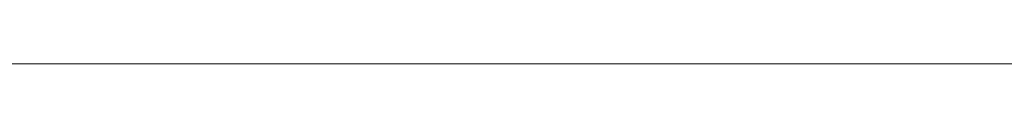
# Model space of a CAD drawing. Units: inches. Extents: x 459864 to 460310, y 324185 to 324787.
# Tile 90 of 112: x 460247.17582 to 460247.24734, y 324283.48323 to 324283.48323. Entities that reach past the tile are written whole.
import ezdxf

# ---------------------------------------------------------------- set-up
doc = ezdxf.new("R2010")
doc.units = ezdxf.units.IN
for name, color, linetype, lineweight in [('A-ANNO-DIMS', 2, 'Continuous', 18), ('L-HRDS', 9, 'Continuous', 18), ('L-SITE-PATT', 252, 'Continuous', 13)]:
    doc.layers.add(name, color=color, linetype=linetype, lineweight=lineweight)
doc.styles.get("Standard").update_dxf_attribs({"font": 'arial.ttf'})
doc.dimstyles.new('ISO-25', dxfattribs={"dimtxt": 6, "dimasz": 2.5, "dimexe": 1.25, "dimexo": 0.625, "dimtad": 1, "dimdec": 1, "dimlunit": 3, "dimtxsty": 'Standard', "dimcen": 2.5, "dimadec": 0, "dimazin": 0, "dimtfac": 1, "dimtdec": 1, "dimtmove": 0, "dimatfit": 3, "dimfxl": 1, "dimarcsym": 0})

# ---------------------------------------------------------------- blocks, each defined once
blk = doc.blocks.new('*D21')
at = {"layer": 'A-ANNO-DIMS', "color": 0, "lineweight": -2, "transparency": 16777216}
for p, q in [((460247.739927, 324715.483233), (460309.580369, 324715.483233)), ((460308.330369, 324712.983233), (460308.330369, 324285.983233)), ((460247.739927, 324283.483233), (460309.580369, 324283.483233))]:
    blk.add_line(p, q, dxfattribs=at)
at = {"layer": 'A-ANNO-DIMS', "color": 0, "transparency": 16777216}
for points in [[(460307.913702, 324712.983233), (460308.747035, 324712.983233), (460308.330369, 324715.483233)], [(460307.913702, 324285.983233), (460308.747035, 324285.983233), (460308.330369, 324283.483233)]]:
    blk.add_solid(points, dxfattribs=at)
at = {"layer": 'Defpoints', "color": 0, "transparency": 16777216}
for p in [(460247.114927, 324715.483233), (460247.114927, 324283.483233), (460308.330369, 324283.483233)]:
    blk.add_point(p, dxfattribs=at)
at = {"layer": 'A-ANNO-DIMS', "color": 0, "transparency": 16777216, "insert": (460304.639884, 324499.483233), "char_height": 6, "attachment_point": 5, "rotation": 90}
blk.add_mtext("36'", dxfattribs=at)

msp = doc.modelspace()

# ---------------------------------------------------------------- hatches: boundary and pattern name
at = {"layer": 'L-SITE-PATT'}
h = msp.add_hatch(dxfattribs=at)
h.set_pattern_fill('DOTS', color=256)
h.paths.add_polyline_path([(460269.803614, 324283.483233), (460247.114927, 324283.483233), (460121.929275, 324283.483233), (460121.929275, 324252.47302), (460117.429275, 324252.47302), (460110.123563, 324252.47302), (460110.123563, 324243.286537), (460080.829543, 324243.286537), (460080.829543, 324252.47302), (460061.114927, 324252.47302), (460061.114927, 324251.882422), (460077.9089, 324251.882422), (460077.9089, 324199.483233), (460080.829543, 324199.483233), (460080.829543, 324207.553216), (460110.123563, 324207.553216), (460110.123563, 324199.483233), (460110.813349, 324199.483233), (460262.114927, 324199.483233), (460269.803614, 324199.483233)], flags=17)
edge = h.paths.add_edge_path(flags=0)
edge.add_ellipse((460222.590295, 324263.813229), major_axis=(-8.485281, 8.485281), ratio=1, start_angle=405, end_angle=495, ccw=False)
edge.add_line((460214.820868, 324254.65989), (460214.831619, 324254.66592))
edge.add_ellipse((460222.590295, 324263.813229), major_axis=(-8.485281, 8.485281), ratio=1, start_angle=405, end_angle=495, ccw=False)
edge.add_line((460210.75891, 324261.780551), (460210.767583, 324261.786823))
edge.add_ellipse((460222.590295, 324263.813229), major_axis=(-8.485281, 8.485281), ratio=1, start_angle=405, end_angle=495, ccw=False)
edge.add_ellipse((460222.590295, 324263.813229), major_axis=(-8.485281, 8.485281), ratio=1, start_angle=392.754016, end_angle=405, ccw=False)
edge.add_ellipse((460222.590295, 324263.813229), major_axis=(-8.485281, 8.485281), ratio=1, start_angle=380.9347178, end_angle=392.754016, ccw=False)
edge.add_line((460211.337059, 324267.985029), (460211.340404, 324267.985029))
edge.add_ellipse((460222.590295, 324263.813229), major_axis=(-8.485281, 8.485281), ratio=1, start_angle=380.9347178, end_angle=392.754016, ccw=False)
edge.add_ellipse((460222.590295, 324263.813229), major_axis=(-8.485281, 8.485281), ratio=1, start_angle=347.9015209, end_angle=380.9347178, ccw=False)
edge.add_ellipse((460222.590295, 324263.813229), major_axis=(-8.485281, 8.485281), ratio=1, start_angle=327.0619241, end_angle=347.9015209, ccw=False)
edge.add_ellipse((460222.590295, 324263.813229), major_axis=(-8.485281, 8.485281), ratio=1, start_angle=278.3246418, end_angle=327.0619241, ccw=False)
edge.add_line((460225.158278, 324275.535991), (460225.157699, 324275.534637))
edge.add_ellipse((460222.590295, 324263.813229), major_axis=(-8.485281, 8.485281), ratio=1, start_angle=278.3246418, end_angle=327.0619241, ccw=False)
edge.add_ellipse((460222.590295, 324263.813229), major_axis=(-8.485281, 8.485281), ratio=1, start_angle=260.6435685, end_angle=278.3246418, ccw=False)
edge.add_ellipse((460222.590295, 324263.813229), major_axis=(-8.485281, 8.485281), ratio=1, start_angle=225, end_angle=260.6435685, ccw=False)
edge.add_line((460234.508791, 324265.242796), (460234.501456, 324265.239441))
edge.add_ellipse((460222.590295, 324263.813229), major_axis=(-8.485281, 8.485281), ratio=1, start_angle=225, end_angle=260.6435685, ccw=False)
edge.add_ellipse((460222.590295, 324263.813229), major_axis=(-8.485281, 8.485281), ratio=1, start_angle=495, end_angle=585, ccw=False)
edge.add_line((460234.436668, 324261.861215), (460234.423783, 324261.857822))
edge.add_ellipse((460222.590295, 324263.813229), major_axis=(-8.485281, 8.485281), ratio=1, start_angle=495, end_angle=585, ccw=False)
edge.add_line((460227.95013, 324253.067192), (460227.946414, 324253.083139))
edge.add_ellipse((460222.590295, 324263.813229), major_axis=(-8.485281, 8.485281), ratio=1, start_angle=495, end_angle=585, ccw=False)
edge.add_line((460226.222975, 324252.369267), (460226.21103, 324252.379551))
edge.add_ellipse((460222.590295, 324263.813229), major_axis=(-8.485281, 8.485281), ratio=1, start_angle=495, end_angle=585, ccw=False)
h.paths.add_polyline_path([(460219.651452, 324254.346654), (460218.461311, 324253.544985), (460218.275437, 324254.78932), (460219.642395, 324256.541765), (460219.62463, 324260.847564), (460216.110089, 324257.333022), (460214.349967, 324256.978066), (460215.416366, 324259.355678), (460212.523935, 324258.495823), (460213.137313, 324259.929797), (460218.507211, 324263.813229), (460222.590295, 324263.813229), (460222.590295, 324267.806698), (460218.175536, 324272.21231), (460219.025968, 324274.63898), (460222.590295, 324272.811129), (460222.590295, 324275.42332), (460223.057099, 324274.824931), (460222.67523, 324273.492211), (460225.911677, 324267.134611), (460219.62463, 324260.847564)], flags=0)
edge = h.paths.add_edge_path(flags=0)
edge.add_ellipse((460194.575758, 324264.046494), major_axis=(-8.485281, 8.485281), ratio=1, start_angle=495, end_angle=585, ccw=False)
edge.add_line((460199.935593, 324253.300458), (460199.931877, 324253.316405))
edge.add_ellipse((460194.575758, 324264.046494), major_axis=(-8.485281, 8.485281), ratio=1, start_angle=495, end_angle=585, ccw=False)
edge.add_line((460198.208438, 324252.602533), (460198.196493, 324252.612817))
edge.add_ellipse((460194.575758, 324264.046494), major_axis=(-8.485281, 8.485281), ratio=1, start_angle=495, end_angle=585, ccw=False)
edge.add_ellipse((460194.575758, 324264.046494), major_axis=(-8.485281, 8.485281), ratio=1, start_angle=405, end_angle=495, ccw=False)
edge.add_line((460186.806331, 324254.893156), (460186.817082, 324254.899186))
edge.add_ellipse((460194.575758, 324264.046494), major_axis=(-8.485281, 8.485281), ratio=1, start_angle=405, end_angle=495, ccw=False)
edge.add_line((460182.744373, 324262.013817), (460182.753046, 324262.020089))
edge.add_ellipse((460194.575758, 324264.046494), major_axis=(-8.485281, 8.485281), ratio=1, start_angle=405, end_angle=495, ccw=False)
edge.add_ellipse((460194.575758, 324264.046494), major_axis=(-8.485281, 8.485281), ratio=1, start_angle=392.754016, end_angle=405, ccw=False)
edge.add_ellipse((460194.575758, 324264.046494), major_axis=(-8.485281, 8.485281), ratio=1, start_angle=380.9347178, end_angle=392.754016, ccw=False)
edge.add_line((460183.322522, 324268.218294), (460183.325867, 324268.218294))
edge.add_ellipse((460194.575758, 324264.046494), major_axis=(-8.485281, 8.485281), ratio=1, start_angle=380.9347178, end_angle=392.754016, ccw=False)
edge.add_ellipse((460194.575758, 324264.046494), major_axis=(-8.485281, 8.485281), ratio=1, start_angle=347.9015209, end_angle=380.9347178, ccw=False)
edge.add_ellipse((460194.575758, 324264.046494), major_axis=(-8.485281, 8.485281), ratio=1, start_angle=327.0619241, end_angle=347.9015209, ccw=False)
edge.add_ellipse((460194.575758, 324264.046494), major_axis=(-8.485281, 8.485281), ratio=1, start_angle=278.3246418, end_angle=327.0619241, ccw=False)
edge.add_line((460197.143741, 324275.769257), (460197.143162, 324275.767903))
edge.add_ellipse((460194.575758, 324264.046494), major_axis=(-8.485281, 8.485281), ratio=1, start_angle=278.3246418, end_angle=327.0619241, ccw=False)
edge.add_ellipse((460194.575758, 324264.046494), major_axis=(-8.485281, 8.485281), ratio=1, start_angle=260.6435685, end_angle=278.3246418, ccw=False)
edge.add_ellipse((460194.575758, 324264.046494), major_axis=(-8.485281, 8.485281), ratio=1, start_angle=225, end_angle=260.6435685, ccw=False)
edge.add_line((460206.494254, 324265.476062), (460206.486919, 324265.472707))
edge.add_ellipse((460194.575758, 324264.046494), major_axis=(-8.485281, 8.485281), ratio=1, start_angle=225, end_angle=260.6435685, ccw=False)
edge.add_ellipse((460194.575758, 324264.046494), major_axis=(-8.485281, 8.485281), ratio=1, start_angle=495, end_angle=585, ccw=False)
edge.add_line((460206.422132, 324262.094481), (460206.409246, 324262.091088))
h.paths.add_polyline_path([(460191.610093, 324261.08083), (460191.636915, 324254.57992), (460190.446774, 324253.778251), (460190.2609, 324255.022585), (460191.627858, 324256.775031), (460191.610093, 324261.08083), (460188.095552, 324257.566288), (460186.33543, 324257.211332), (460187.40183, 324259.588944), (460184.509398, 324258.729088), (460185.122776, 324260.163063), (460190.492675, 324264.046494), (460194.575758, 324264.046494), (460194.575758, 324268.039963), (460190.160999, 324272.445576), (460191.011431, 324274.872246), (460194.575758, 324273.044395), (460194.575758, 324275.656585), (460195.042562, 324275.058197), (460194.660693, 324273.725477), (460197.897141, 324267.367877)], flags=0)
edge = h.paths.add_edge_path(flags=0)
edge.add_ellipse((460252.911961, 324263.577616), major_axis=(-8.485281, 8.485281), ratio=1, start_angle=405, end_angle=495, ccw=False)
edge.add_line((460241.080576, 324261.544938), (460241.089249, 324261.55121))
edge.add_ellipse((460252.911961, 324263.577616), major_axis=(-8.485281, 8.485281), ratio=1, start_angle=405, end_angle=495, ccw=False)
edge.add_ellipse((460252.911961, 324263.577616), major_axis=(-8.485281, 8.485281), ratio=1, start_angle=392.754016, end_angle=405, ccw=False)
edge.add_ellipse((460252.911961, 324263.577616), major_axis=(-8.485281, 8.485281), ratio=1, start_angle=380.9347178, end_angle=392.754016, ccw=False)
edge.add_line((460241.658725, 324267.749416), (460241.66207, 324267.749416))
edge.add_ellipse((460252.911961, 324263.577616), major_axis=(-8.485281, 8.485281), ratio=1, start_angle=380.9347178, end_angle=392.754016, ccw=False)
edge.add_ellipse((460252.911961, 324263.577616), major_axis=(-8.485281, 8.485281), ratio=1, start_angle=347.9015209, end_angle=380.9347178, ccw=False)
edge.add_ellipse((460252.911961, 324263.577616), major_axis=(-8.485281, 8.485281), ratio=1, start_angle=327.0619241, end_angle=347.9015209, ccw=False)
edge.add_ellipse((460252.911961, 324263.577616), major_axis=(-8.485281, 8.485281), ratio=1, start_angle=278.3246418, end_angle=327.0619241, ccw=False)
edge.add_line((460255.479944, 324275.300378), (460255.479365, 324275.299024))
edge.add_ellipse((460252.911961, 324263.577616), major_axis=(-8.485281, 8.485281), ratio=1, start_angle=278.3246418, end_angle=327.0619241, ccw=False)
edge.add_ellipse((460252.911961, 324263.577616), major_axis=(-8.485281, 8.485281), ratio=1, start_angle=260.6435685, end_angle=278.3246418, ccw=False)
edge.add_ellipse((460252.911961, 324263.577616), major_axis=(-8.485281, 8.485281), ratio=1, start_angle=225, end_angle=260.6435685, ccw=False)
edge.add_line((460264.830457, 324265.007183), (460264.823122, 324265.003828))
edge.add_ellipse((460252.911961, 324263.577616), major_axis=(-8.485281, 8.485281), ratio=1, start_angle=225, end_angle=260.6435685, ccw=False)
edge.add_ellipse((460252.911961, 324263.577616), major_axis=(-8.485281, 8.485281), ratio=1, start_angle=495, end_angle=585, ccw=False)
edge.add_line((460264.758335, 324261.625602), (460264.745449, 324261.622209))
edge.add_ellipse((460252.911961, 324263.577616), major_axis=(-8.485281, 8.485281), ratio=1, start_angle=495, end_angle=585, ccw=False)
edge.add_line((460258.271796, 324252.831579), (460258.268081, 324252.847526))
edge.add_ellipse((460252.911961, 324263.577616), major_axis=(-8.485281, 8.485281), ratio=1, start_angle=495, end_angle=585, ccw=False)
edge.add_line((460256.544641, 324252.133654), (460256.532696, 324252.143938))
edge.add_ellipse((460252.911961, 324263.577616), major_axis=(-8.485281, 8.485281), ratio=1, start_angle=495, end_angle=585, ccw=False)
edge.add_ellipse((460252.911961, 324263.577616), major_axis=(-8.485281, 8.485281), ratio=1, start_angle=405, end_angle=495, ccw=False)
edge.add_line((460245.142534, 324254.424277), (460245.153285, 324254.430307))
h.paths.add_polyline_path([(460244.671633, 324256.742453), (460245.738033, 324259.120065), (460242.845601, 324258.26021), (460243.458979, 324259.694184), (460248.828878, 324263.577616), (460252.911961, 324263.577616), (460252.911961, 324267.571085), (460248.497202, 324271.976697), (460249.347634, 324274.403367), (460252.911961, 324272.575516), (460252.911961, 324275.187707), (460253.378765, 324274.589318), (460252.996897, 324273.256598), (460256.233344, 324266.898998), (460249.946296, 324260.611951), (460249.973118, 324254.111041), (460248.782977, 324253.309372), (460248.597103, 324254.553707), (460249.964061, 324256.306152), (460249.946296, 324260.611951), (460246.431755, 324257.097409)], flags=0)
edge = h.paths.add_edge_path(flags=0)
edge.add_ellipse((460167.43869, 324262.832792), major_axis=(-8.485281, 8.485281), ratio=1, start_angle=495, end_angle=585, ccw=False)
edge.add_line((460172.798524, 324252.086755), (460172.794809, 324252.102702))
edge.add_ellipse((460167.43869, 324262.832792), major_axis=(-8.485281, 8.485281), ratio=1, start_angle=495, end_angle=585, ccw=False)
edge.add_line((460171.07137, 324251.38883), (460171.059425, 324251.399114))
edge.add_ellipse((460167.43869, 324262.832792), major_axis=(-8.485281, 8.485281), ratio=1, start_angle=495, end_angle=585, ccw=False)
edge.add_ellipse((460167.43869, 324262.832792), major_axis=(-8.485281, 8.485281), ratio=1, start_angle=405, end_angle=495, ccw=False)
edge.add_line((460159.669262, 324253.679453), (460159.680013, 324253.685483))
edge.add_ellipse((460167.43869, 324262.832792), major_axis=(-8.485281, 8.485281), ratio=1, start_angle=405, end_angle=495, ccw=False)
edge.add_line((460155.607304, 324260.800114), (460155.615977, 324260.806386))
edge.add_ellipse((460167.43869, 324262.832792), major_axis=(-8.485281, 8.485281), ratio=1, start_angle=405, end_angle=495, ccw=False)
edge.add_ellipse((460167.43869, 324262.832792), major_axis=(-8.485281, 8.485281), ratio=1, start_angle=392.754016, end_angle=405, ccw=False)
edge.add_ellipse((460167.43869, 324262.832792), major_axis=(-8.485281, 8.485281), ratio=1, start_angle=380.9347178, end_angle=392.754016, ccw=False)
edge.add_line((460156.185453, 324267.004592), (460156.188798, 324267.004592))
edge.add_ellipse((460167.43869, 324262.832792), major_axis=(-8.485281, 8.485281), ratio=1, start_angle=380.9347178, end_angle=392.754016, ccw=False)
edge.add_ellipse((460167.43869, 324262.832792), major_axis=(-8.485281, 8.485281), ratio=1, start_angle=347.9015209, end_angle=380.9347178, ccw=False)
edge.add_ellipse((460167.43869, 324262.832792), major_axis=(-8.485281, 8.485281), ratio=1, start_angle=327.0619241, end_angle=347.9015209, ccw=False)
edge.add_ellipse((460167.43869, 324262.832792), major_axis=(-8.485281, 8.485281), ratio=1, start_angle=278.3246418, end_angle=327.0619241, ccw=False)
edge.add_line((460170.006672, 324274.555554), (460170.006093, 324274.5542))
edge.add_ellipse((460167.43869, 324262.832792), major_axis=(-8.485281, 8.485281), ratio=1, start_angle=278.3246418, end_angle=327.0619241, ccw=False)
edge.add_ellipse((460167.43869, 324262.832792), major_axis=(-8.485281, 8.485281), ratio=1, start_angle=260.6435685, end_angle=278.3246418, ccw=False)
edge.add_ellipse((460167.43869, 324262.832792), major_axis=(-8.485281, 8.485281), ratio=1, start_angle=225, end_angle=260.6435685, ccw=False)
edge.add_line((460179.357186, 324264.262359), (460179.349851, 324264.259004))
edge.add_ellipse((460167.43869, 324262.832792), major_axis=(-8.485281, 8.485281), ratio=1, start_angle=225, end_angle=260.6435685, ccw=False)
edge.add_ellipse((460167.43869, 324262.832792), major_axis=(-8.485281, 8.485281), ratio=1, start_angle=495, end_angle=585, ccw=False)
edge.add_line((460179.285063, 324260.880778), (460179.272177, 324260.877385))
h.paths.add_polyline_path([(460164.473025, 324259.867127), (460164.499846, 324253.366217), (460163.309706, 324252.564548), (460163.123831, 324253.808883), (460164.49079, 324255.561328), (460164.473025, 324259.867127), (460160.958483, 324256.352585), (460159.198362, 324255.997629), (460160.264761, 324258.375241), (460157.372329, 324257.515386), (460157.985707, 324258.94936), (460163.355606, 324262.832792), (460167.43869, 324262.832792), (460167.43869, 324266.826261), (460163.02393, 324271.231873), (460163.874362, 324273.658543), (460167.43869, 324271.830692), (460167.43869, 324274.442883), (460167.905493, 324273.844494), (460167.523625, 324272.511774), (460170.760072, 324266.154174)], flags=0)
edge = h.paths.add_edge_path(flags=0)
edge.add_ellipse((460140.758089, 324262.369585), major_axis=(-8.485281, 8.485281), ratio=1, start_angle=495, end_angle=585, ccw=False)
edge.add_line((460146.117923, 324251.623548), (460146.114208, 324251.639495))
edge.add_ellipse((460140.758089, 324262.369585), major_axis=(-8.485281, 8.485281), ratio=1, start_angle=495, end_angle=585, ccw=False)
edge.add_line((460144.390769, 324250.925623), (460144.378824, 324250.935907))
edge.add_ellipse((460140.758089, 324262.369585), major_axis=(-8.485281, 8.485281), ratio=1, start_angle=495, end_angle=585, ccw=False)
edge.add_ellipse((460140.758089, 324262.369585), major_axis=(-8.485281, 8.485281), ratio=1, start_angle=405, end_angle=495, ccw=False)
edge.add_line((460132.988661, 324253.216246), (460132.999412, 324253.222276))
edge.add_ellipse((460140.758089, 324262.369585), major_axis=(-8.485281, 8.485281), ratio=1, start_angle=405, end_angle=495, ccw=False)
edge.add_line((460128.926703, 324260.336907), (460128.935376, 324260.343179))
edge.add_ellipse((460140.758089, 324262.369585), major_axis=(-8.485281, 8.485281), ratio=1, start_angle=405, end_angle=495, ccw=False)
edge.add_ellipse((460140.758089, 324262.369585), major_axis=(-8.485281, 8.485281), ratio=1, start_angle=392.754016, end_angle=405, ccw=False)
edge.add_ellipse((460140.758089, 324262.369585), major_axis=(-8.485281, 8.485281), ratio=1, start_angle=380.9347178, end_angle=392.754016, ccw=False)
edge.add_line((460129.504852, 324266.541385), (460129.508197, 324266.541385))
edge.add_ellipse((460140.758089, 324262.369585), major_axis=(-8.485281, 8.485281), ratio=1, start_angle=380.9347178, end_angle=392.754016, ccw=False)
edge.add_ellipse((460140.758089, 324262.369585), major_axis=(-8.485281, 8.485281), ratio=1, start_angle=347.9015209, end_angle=380.9347178, ccw=False)
edge.add_ellipse((460140.758089, 324262.369585), major_axis=(-8.485281, 8.485281), ratio=1, start_angle=327.0619241, end_angle=347.9015209, ccw=False)
edge.add_ellipse((460140.758089, 324262.369585), major_axis=(-8.485281, 8.485281), ratio=1, start_angle=278.3246418, end_angle=327.0619241, ccw=False)
edge.add_line((460143.326071, 324274.092347), (460143.325492, 324274.090993))
edge.add_ellipse((460140.758089, 324262.369585), major_axis=(-8.485281, 8.485281), ratio=1, start_angle=278.3246418, end_angle=327.0619241, ccw=False)
edge.add_ellipse((460140.758089, 324262.369585), major_axis=(-8.485281, 8.485281), ratio=1, start_angle=260.6435685, end_angle=278.3246418, ccw=False)
edge.add_ellipse((460140.758089, 324262.369585), major_axis=(-8.485281, 8.485281), ratio=1, start_angle=225, end_angle=260.6435685, ccw=False)
edge.add_line((460152.676585, 324263.799152), (460152.66925, 324263.795797))
edge.add_ellipse((460140.758089, 324262.369585), major_axis=(-8.485281, 8.485281), ratio=1, start_angle=225, end_angle=260.6435685, ccw=False)
edge.add_ellipse((460140.758089, 324262.369585), major_axis=(-8.485281, 8.485281), ratio=1, start_angle=495, end_angle=585, ccw=False)
edge.add_line((460152.604462, 324260.417571), (460152.591576, 324260.414178))
h.paths.add_polyline_path([(460137.792424, 324259.40392), (460137.819245, 324252.90301), (460136.629105, 324252.101341), (460136.44323, 324253.345676), (460137.810189, 324255.098121), (460137.792424, 324259.40392), (460134.277882, 324255.889378), (460132.517761, 324255.534422), (460133.58416, 324257.912034), (460130.691728, 324257.052179), (460131.305106, 324258.486153), (460136.675005, 324262.369585), (460140.758089, 324262.369585), (460140.758089, 324266.363054), (460136.343329, 324270.768666), (460137.193761, 324273.195336), (460140.758089, 324271.367485), (460140.758089, 324273.979676), (460141.224892, 324273.381287), (460140.843024, 324272.048567), (460144.079471, 324265.690967)], flags=0)
h.paths.add_polyline_path([(460110.123563, 324227.413868), (460080.829543, 324227.413868), (460080.829543, 324235.483851), (460110.123563, 324235.483851)], flags=16)
h.paths.add_polyline_path([(460110.123563, 324220.796634), (460110.123563, 324212.726651), (460080.829543, 324212.726651), (460080.829543, 324220.796634)], flags=16)
h.paths.add_polyline_path([(460269.803614, 324283.483233), (460247.114927, 324283.483233), (460121.929275, 324283.483233), (460121.929275, 324252.47302), (460117.429275, 324252.47302), (460110.123563, 324252.47302), (460110.123563, 324243.286537), (460080.829543, 324243.286537), (460080.829543, 324252.47302), (460061.114927, 324252.47302), (460061.114927, 324251.882422), (460077.9089, 324251.882422), (460077.9089, 324199.483233), (460080.829543, 324199.483233), (460080.829543, 324207.553216), (460110.123563, 324207.553216), (460110.123563, 324199.483233), (460262.114927, 324199.483233), (460269.803614, 324199.483233)], flags=17)
h.paths.add_polyline_path([(460219.651452, 324254.346654), (460218.461311, 324253.544985), (460218.275437, 324254.78932), (460219.642395, 324256.541765), (460219.62463, 324260.847564), (460216.110089, 324257.333022), (460214.349967, 324256.978066), (460215.416366, 324259.355678), (460212.523935, 324258.495823), (460213.137313, 324259.929797), (460218.507211, 324263.813229), (460222.590295, 324263.813229), (460220.180486, 324266.223037), (460215.460959, 324265.307646), (460211.834533, 324266.136551), (460216.246619, 324267.985029), (460218.418495, 324267.985029), (460222.590295, 324263.813229), (460222.590295, 324267.806698), (460218.175536, 324272.21231), (460219.025968, 324274.63898), (460222.590295, 324272.811129), (460222.590295, 324275.42332), (460223.057099, 324274.824931), (460222.67523, 324273.492211), (460225.911677, 324267.134611), (460222.590295, 324263.813229), (460231.382871, 324263.813229), (460228.484718, 324262.487825), (460224.425208, 324261.978316), (460228.679899, 324257.723625), (460228.965835, 324254.791014), (460227.141768, 324256.536632), (460227.542067, 324254.818575), (460227.333342, 324253.614466), (460222.590295, 324259.984626), (460222.590295, 324255.496666), (460221.377409, 324256.540849), (460220.575794, 324261.798728), (460219.62463, 324260.847564)], flags=0)
h.paths.add_polyline_path([(460199.127231, 324256.769898), (460199.52753, 324255.051841), (460199.318805, 324253.847732), (460194.575758, 324260.217892), (460194.575758, 324255.729932), (460193.362872, 324256.774115), (460192.561257, 324262.031993), (460191.610093, 324261.08083), (460191.636915, 324254.57992), (460190.446774, 324253.778251), (460190.2609, 324255.022585), (460191.627858, 324256.775031), (460191.610093, 324261.08083), (460188.095552, 324257.566288), (460186.33543, 324257.211332), (460187.40183, 324259.588944), (460184.509398, 324258.729088), (460185.122776, 324260.163063), (460190.492675, 324264.046494), (460194.575758, 324264.046494), (460192.16595, 324266.456303), (460187.446422, 324265.540912), (460183.819996, 324266.369816), (460188.232082, 324268.218294), (460190.403958, 324268.218294), (460194.575758, 324264.046494), (460194.575758, 324268.039963), (460190.160999, 324272.445576), (460191.011431, 324274.872246), (460194.575758, 324273.044395), (460194.575758, 324275.656585), (460195.042562, 324275.058197), (460194.660693, 324273.725477), (460197.897141, 324267.367877), (460194.575758, 324264.046494), (460203.368334, 324264.046494), (460200.470181, 324262.721091), (460196.410671, 324262.211582), (460200.665362, 324257.956891), (460200.951298, 324255.02428)], flags=0)
h.paths.add_polyline_path([(460244.671633, 324256.742453), (460245.738033, 324259.120065), (460242.845601, 324258.26021), (460243.458979, 324259.694184), (460248.828878, 324263.577616), (460252.911961, 324263.577616), (460250.502153, 324265.987424), (460245.782625, 324265.072033), (460242.156199, 324265.900938), (460246.568285, 324267.749416), (460248.740161, 324267.749416), (460252.911961, 324263.577616), (460252.911961, 324267.571085), (460248.497202, 324271.976697), (460249.347634, 324274.403367), (460252.911961, 324272.575516), (460252.911961, 324275.187707), (460253.378765, 324274.589318), (460252.996897, 324273.256598), (460256.233344, 324266.898998), (460252.911961, 324263.577616), (460261.704537, 324263.577616), (460258.806384, 324262.252212), (460254.746874, 324261.742703), (460259.001565, 324257.488012), (460259.287501, 324254.555401), (460257.463434, 324256.301019), (460257.863733, 324254.582962), (460257.655008, 324253.378853), (460252.911961, 324259.749013), (460252.911961, 324255.261053), (460251.699075, 324256.305236), (460250.89746, 324261.563115), (460249.946296, 324260.611951), (460249.973118, 324254.111041), (460248.782977, 324253.309372), (460248.597103, 324254.553707), (460249.964061, 324256.306152), (460249.946296, 324260.611951), (460246.431755, 324257.097409)], flags=0)
h.paths.add_polyline_path([(460173.528293, 324256.743188), (460173.81423, 324253.810577), (460171.990163, 324255.556195), (460172.390461, 324253.838138), (460172.181736, 324252.634029), (460167.43869, 324259.004189), (460167.43869, 324254.516229), (460166.225803, 324255.560412), (460165.424189, 324260.818291), (460164.473025, 324259.867127), (460164.499846, 324253.366217), (460163.309706, 324252.564548), (460163.123831, 324253.808883), (460164.49079, 324255.561328), (460164.473025, 324259.867127), (460160.958483, 324256.352585), (460159.198362, 324255.997629), (460160.264761, 324258.375241), (460157.372329, 324257.515386), (460157.985707, 324258.94936), (460163.355606, 324262.832792), (460167.43869, 324262.832792), (460165.028881, 324265.2426), (460160.309353, 324264.327209), (460156.682927, 324265.156114), (460161.095013, 324267.004592), (460163.26689, 324267.004592), (460167.43869, 324262.832792), (460167.43869, 324266.826261), (460163.02393, 324271.231873), (460163.874362, 324273.658543), (460167.43869, 324271.830692), (460167.43869, 324274.442883), (460167.905493, 324273.844494), (460167.523625, 324272.511774), (460170.760072, 324266.154174), (460167.43869, 324262.832792), (460176.231266, 324262.832792), (460173.333113, 324261.507388), (460169.273603, 324260.997879)], flags=0)
h.paths.add_polyline_path([(460146.847692, 324256.279981), (460147.133629, 324253.34737), (460145.309562, 324255.092988), (460145.70986, 324253.374931), (460145.501135, 324252.170822), (460140.758089, 324258.540983), (460140.758089, 324254.053022), (460139.545202, 324255.097205), (460138.743588, 324260.355084), (460137.792424, 324259.40392), (460137.819245, 324252.90301), (460136.629105, 324252.101341), (460136.44323, 324253.345676), (460137.810189, 324255.098121), (460137.792424, 324259.40392), (460134.277882, 324255.889378), (460132.517761, 324255.534422), (460133.58416, 324257.912034), (460130.691728, 324257.052179), (460131.305106, 324258.486153), (460136.675005, 324262.369585), (460140.758089, 324262.369585), (460138.34828, 324264.779393), (460133.628752, 324263.864002), (460130.002326, 324264.692907), (460134.414412, 324266.541385), (460136.586289, 324266.541385), (460140.758089, 324262.369585), (460140.758089, 324266.363054), (460136.343329, 324270.768666), (460137.193761, 324273.195336), (460140.758089, 324271.367485), (460140.758089, 324273.979676), (460141.224892, 324273.381287), (460140.843024, 324272.048567), (460144.079471, 324265.690967), (460140.758089, 324262.369585), (460149.550664, 324262.369585), (460146.652512, 324261.044182), (460142.593002, 324260.534672)], flags=0)
edge = h.paths.add_edge_path()
edge.add_line((460269.803614, 324272.549054), (460260.881484, 324272.549054))
edge.add_ellipse((460252.911961, 324263.577616), major_axis=(-8.485281, 8.485281), ratio=1, start_angle=260.6435685, end_angle=273.3846244, ccw=False)
edge.add_line((460262.282614, 324271.092108), (460262.260554, 324271.09106))
edge.add_ellipse((460252.911961, 324263.577616), major_axis=(-8.485281, 8.485281), ratio=1, start_angle=260.6435685, end_angle=273.3846244, ccw=False)
edge.add_ellipse((460252.911961, 324263.577616), major_axis=(-8.485281, 8.485281), ratio=1, start_angle=225, end_angle=260.6435685, ccw=False)
edge.add_line((460263.608568, 324269.063294), (460263.571652, 324269.058283))
edge.add_ellipse((460252.911961, 324263.577616), major_axis=(-8.485281, 8.485281), ratio=1, start_angle=225, end_angle=260.6435685, ccw=False)
edge.add_line((460264.615462, 324266.30554), (460264.585358, 324266.305196))
edge.add_ellipse((460252.911961, 324263.577616), major_axis=(-8.485281, 8.485281), ratio=1, start_angle=225, end_angle=260.6435685, ccw=False)
edge.add_line((460264.830457, 324265.007183), (460264.823122, 324265.003828))
edge.add_ellipse((460252.911961, 324263.577616), major_axis=(-8.485281, 8.485281), ratio=1, start_angle=225, end_angle=260.6435685, ccw=False)
edge.add_ellipse((460252.911961, 324263.577616), major_axis=(-8.485281, 8.485281), ratio=1, start_angle=495, end_angle=585, ccw=False)
edge.add_line((460264.758335, 324261.625602), (460264.745449, 324261.622209))
edge.add_ellipse((460252.911961, 324263.577616), major_axis=(-8.485281, 8.485281), ratio=1, start_angle=495, end_angle=585, ccw=False)
edge.add_line((460263.442202, 324257.739018), (460263.389259, 324257.779239))
edge.add_ellipse((460252.911961, 324263.577616), major_axis=(-8.485281, 8.485281), ratio=1, start_angle=495, end_angle=585, ccw=False)
edge.add_line((460258.128071, 324252.743505), (460258.101878, 324252.778683))
edge.add_ellipse((460252.911961, 324263.577616), major_axis=(-8.485281, 8.485281), ratio=1, start_angle=495, end_angle=585, ccw=False)
edge.add_line((460256.544641, 324252.133654), (460256.532696, 324252.143938))
edge.add_ellipse((460252.911961, 324263.577616), major_axis=(-8.485281, 8.485281), ratio=1, start_angle=495, end_angle=585, ccw=False)
edge.add_ellipse((460252.911961, 324263.577616), major_axis=(-8.485281, 8.485281), ratio=1, start_angle=405, end_angle=495, ccw=False)
edge.add_line((460250.593989, 324251.780412), (460250.604653, 324251.819817))
edge.add_ellipse((460252.911961, 324263.577616), major_axis=(-8.485281, 8.485281), ratio=1, start_angle=405, end_angle=495, ccw=False)
edge.add_line((460245.142534, 324254.424277), (460245.153285, 324254.430307))
edge.add_ellipse((460252.911961, 324263.577616), major_axis=(-8.485281, 8.485281), ratio=1, start_angle=405, end_angle=495, ccw=False)
edge.add_line((460243.524588, 324256.059004), (460243.560343, 324256.091361))
edge.add_ellipse((460252.911961, 324263.577616), major_axis=(-8.485281, 8.485281), ratio=1, start_angle=405, end_angle=495, ccw=False)
edge.add_line((460241.440103, 324259.892726), (460241.522441, 324259.895877))
edge.add_ellipse((460252.911961, 324263.577616), major_axis=(-8.485281, 8.485281), ratio=1, start_angle=405, end_angle=495, ccw=False)
edge.add_line((460241.080576, 324261.544938), (460241.089249, 324261.55121))
edge.add_ellipse((460252.911961, 324263.577616), major_axis=(-8.485281, 8.485281), ratio=1, start_angle=405, end_angle=495, ccw=False)
edge.add_ellipse((460252.911961, 324263.577616), major_axis=(-8.485281, 8.485281), ratio=1, start_angle=392.754016, end_angle=405, ccw=False)
edge.add_line((460241.050299, 324265.437612), (460241.062566, 324265.442751))
edge.add_ellipse((460252.911961, 324263.577616), major_axis=(-8.485281, 8.485281), ratio=1, start_angle=392.754016, end_angle=405, ccw=False)
edge.add_ellipse((460252.911961, 324263.577616), major_axis=(-8.485281, 8.485281), ratio=1, start_angle=380.9347178, end_angle=392.754016, ccw=False)
edge.add_line((460241.451888, 324267.176391), (460241.469044, 324267.170988))
edge.add_ellipse((460252.911961, 324263.577616), major_axis=(-8.485281, 8.485281), ratio=1, start_angle=380.9347178, end_angle=392.754016, ccw=False)
edge.add_line((460241.658725, 324267.749416), (460241.66207, 324267.749416))
edge.add_ellipse((460252.911961, 324263.577616), major_axis=(-8.485281, 8.485281), ratio=1, start_angle=380.9347178, end_angle=392.754016, ccw=False)
edge.add_ellipse((460252.911961, 324263.577616), major_axis=(-8.485281, 8.485281), ratio=1, start_angle=356.6153756, end_angle=380.9347178, ccw=False)
edge.add_line((460244.880293, 324272.487651), (460244.712651, 324272.549054))
edge.add_line((460244.712651, 324272.549054), (460230.817406, 324272.549054))
edge.add_ellipse((460222.590295, 324263.813229), major_axis=(-8.485281, 8.485281), ratio=1, start_angle=260.6435685, end_angle=271.7177746, ccw=False)
edge.add_ellipse((460222.590295, 324263.813229), major_axis=(-8.485281, 8.485281), ratio=1, start_angle=225, end_angle=260.6435685, ccw=False)
edge.add_line((460233.286902, 324269.298907), (460233.249986, 324269.293896))
edge.add_ellipse((460222.590295, 324263.813229), major_axis=(-8.485281, 8.485281), ratio=1, start_angle=225, end_angle=260.6435685, ccw=False)
edge.add_line((460234.293796, 324266.541153), (460234.263692, 324266.540809))
edge.add_ellipse((460222.590295, 324263.813229), major_axis=(-8.485281, 8.485281), ratio=1, start_angle=225, end_angle=260.6435685, ccw=False)
edge.add_line((460234.508791, 324265.242796), (460234.501456, 324265.239441))
edge.add_ellipse((460222.590295, 324263.813229), major_axis=(-8.485281, 8.485281), ratio=1, start_angle=225, end_angle=260.6435685, ccw=False)
edge.add_ellipse((460222.590295, 324263.813229), major_axis=(-8.485281, 8.485281), ratio=1, start_angle=495, end_angle=585, ccw=False)
edge.add_line((460234.436668, 324261.861215), (460234.423783, 324261.857822))
edge.add_ellipse((460222.590295, 324263.813229), major_axis=(-8.485281, 8.485281), ratio=1, start_angle=495, end_angle=585, ccw=False)
edge.add_line((460233.120535, 324257.974631), (460233.067593, 324258.014852))
edge.add_ellipse((460222.590295, 324263.813229), major_axis=(-8.485281, 8.485281), ratio=1, start_angle=495, end_angle=585, ccw=False)
edge.add_line((460227.806405, 324252.979118), (460227.780212, 324253.014296))
edge.add_ellipse((460222.590295, 324263.813229), major_axis=(-8.485281, 8.485281), ratio=1, start_angle=495, end_angle=585, ccw=False)
edge.add_line((460226.222975, 324252.369267), (460226.21103, 324252.379551))
edge.add_ellipse((460222.590295, 324263.813229), major_axis=(-8.485281, 8.485281), ratio=1, start_angle=495, end_angle=585, ccw=False)
edge.add_ellipse((460222.590295, 324263.813229), major_axis=(-8.485281, 8.485281), ratio=1, start_angle=405, end_angle=495, ccw=False)
edge.add_line((460220.272323, 324252.016025), (460220.282987, 324252.05543))
edge.add_ellipse((460222.590295, 324263.813229), major_axis=(-8.485281, 8.485281), ratio=1, start_angle=405, end_angle=495, ccw=False)
edge.add_line((460214.820868, 324254.65989), (460214.831619, 324254.66592))
edge.add_ellipse((460222.590295, 324263.813229), major_axis=(-8.485281, 8.485281), ratio=1, start_angle=405, end_angle=495, ccw=False)
edge.add_line((460213.202922, 324256.294617), (460213.238677, 324256.326974))
edge.add_ellipse((460222.590295, 324263.813229), major_axis=(-8.485281, 8.485281), ratio=1, start_angle=405, end_angle=495, ccw=False)
edge.add_line((460211.118437, 324260.128339), (460211.200774, 324260.13149))
edge.add_ellipse((460222.590295, 324263.813229), major_axis=(-8.485281, 8.485281), ratio=1, start_angle=405, end_angle=495, ccw=False)
edge.add_line((460210.75891, 324261.780551), (460210.767583, 324261.786823))
edge.add_ellipse((460222.590295, 324263.813229), major_axis=(-8.485281, 8.485281), ratio=1, start_angle=405, end_angle=495, ccw=False)
edge.add_ellipse((460222.590295, 324263.813229), major_axis=(-8.485281, 8.485281), ratio=1, start_angle=392.754016, end_angle=405, ccw=False)
edge.add_line((460210.728633, 324265.673225), (460210.7409, 324265.678364))
edge.add_ellipse((460222.590295, 324263.813229), major_axis=(-8.485281, 8.485281), ratio=1, start_angle=392.754016, end_angle=405, ccw=False)
edge.add_ellipse((460222.590295, 324263.813229), major_axis=(-8.485281, 8.485281), ratio=1, start_angle=380.9347178, end_angle=392.754016, ccw=False)
edge.add_line((460211.130222, 324267.412004), (460211.147378, 324267.406601))
edge.add_ellipse((460222.590295, 324263.813229), major_axis=(-8.485281, 8.485281), ratio=1, start_angle=380.9347178, end_angle=392.754016, ccw=False)
edge.add_line((460211.337059, 324267.985029), (460211.340404, 324267.985029))
edge.add_ellipse((460222.590295, 324263.813229), major_axis=(-8.485281, 8.485281), ratio=1, start_angle=380.9347178, end_angle=392.754016, ccw=False)
edge.add_ellipse((460222.590295, 324263.813229), major_axis=(-8.485281, 8.485281), ratio=1, start_angle=358.2822254, end_angle=380.9347178, ccw=False)
edge.add_line((460213.704522, 324271.901826), (460213.709044, 324271.868974))
edge.add_ellipse((460222.590295, 324263.813229), major_axis=(-8.485281, 8.485281), ratio=1, start_angle=358.2822254, end_angle=380.9347178, ccw=False)
edge.add_line((460214.363185, 324272.549054), (460203.078318, 324272.549054))
edge.add_line((460203.078318, 324272.549054), (460203.060342, 324272.531078))
edge.add_ellipse((460194.575758, 324264.046494), major_axis=(-8.485281, 8.485281), ratio=1, start_angle=260.6435685, end_angle=270.11679, ccw=False)
edge.add_line((460203.956591, 324271.56147), (460203.920907, 324271.559776))
edge.add_ellipse((460194.575758, 324264.046494), major_axis=(-8.485281, 8.485281), ratio=1, start_angle=260.6435685, end_angle=270.11679, ccw=False)
edge.add_ellipse((460194.575758, 324264.046494), major_axis=(-8.485281, 8.485281), ratio=1, start_angle=225, end_angle=260.6435685, ccw=False)
edge.add_line((460205.272365, 324269.532172), (460205.235449, 324269.527161))
edge.add_ellipse((460194.575758, 324264.046494), major_axis=(-8.485281, 8.485281), ratio=1, start_angle=225, end_angle=260.6435685, ccw=False)
edge.add_line((460206.279259, 324266.774419), (460206.249155, 324266.774075))
edge.add_ellipse((460194.575758, 324264.046494), major_axis=(-8.485281, 8.485281), ratio=1, start_angle=225, end_angle=260.6435685, ccw=False)
edge.add_line((460206.494254, 324265.476062), (460206.486919, 324265.472707))
edge.add_ellipse((460194.575758, 324264.046494), major_axis=(-8.485281, 8.485281), ratio=1, start_angle=225, end_angle=260.6435685, ccw=False)
edge.add_ellipse((460194.575758, 324264.046494), major_axis=(-8.485281, 8.485281), ratio=1, start_angle=495, end_angle=585, ccw=False)
edge.add_line((460206.422132, 324262.094481), (460206.409246, 324262.091088))
edge.add_ellipse((460194.575758, 324264.046494), major_axis=(-8.485281, 8.485281), ratio=1, start_angle=495, end_angle=585, ccw=False)
edge.add_line((460205.105999, 324258.207897), (460205.053056, 324258.248118))
edge.add_ellipse((460194.575758, 324264.046494), major_axis=(-8.485281, 8.485281), ratio=1, start_angle=495, end_angle=585, ccw=False)
edge.add_line((460199.791868, 324253.212383), (460199.765675, 324253.247562))
edge.add_ellipse((460194.575758, 324264.046494), major_axis=(-8.485281, 8.485281), ratio=1, start_angle=495, end_angle=585, ccw=False)
edge.add_line((460198.208438, 324252.602533), (460198.196493, 324252.612817))
edge.add_ellipse((460194.575758, 324264.046494), major_axis=(-8.485281, 8.485281), ratio=1, start_angle=495, end_angle=585, ccw=False)
edge.add_ellipse((460194.575758, 324264.046494), major_axis=(-8.485281, 8.485281), ratio=1, start_angle=405, end_angle=495, ccw=False)
edge.add_line((460192.257786, 324252.249291), (460192.26845, 324252.288696))
edge.add_ellipse((460194.575758, 324264.046494), major_axis=(-8.485281, 8.485281), ratio=1, start_angle=405, end_angle=495, ccw=False)
edge.add_line((460186.806331, 324254.893156), (460186.817082, 324254.899186))
edge.add_ellipse((460194.575758, 324264.046494), major_axis=(-8.485281, 8.485281), ratio=1, start_angle=405, end_angle=495, ccw=False)
edge.add_line((460185.188385, 324256.527883), (460185.22414, 324256.56024))
edge.add_ellipse((460194.575758, 324264.046494), major_axis=(-8.485281, 8.485281), ratio=1, start_angle=405, end_angle=495, ccw=False)
edge.add_line((460183.1039, 324260.361604), (460183.186238, 324260.364755))
edge.add_ellipse((460194.575758, 324264.046494), major_axis=(-8.485281, 8.485281), ratio=1, start_angle=405, end_angle=495, ccw=False)
edge.add_line((460182.744373, 324262.013817), (460182.753046, 324262.020089))
edge.add_ellipse((460194.575758, 324264.046494), major_axis=(-8.485281, 8.485281), ratio=1, start_angle=405, end_angle=495, ccw=False)
edge.add_ellipse((460194.575758, 324264.046494), major_axis=(-8.485281, 8.485281), ratio=1, start_angle=392.754016, end_angle=405, ccw=False)
edge.add_line((460182.714096, 324265.906491), (460182.726363, 324265.91163))
edge.add_ellipse((460194.575758, 324264.046494), major_axis=(-8.485281, 8.485281), ratio=1, start_angle=392.754016, end_angle=405, ccw=False)
edge.add_ellipse((460194.575758, 324264.046494), major_axis=(-8.485281, 8.485281), ratio=1, start_angle=380.9347178, end_angle=392.754016, ccw=False)
edge.add_line((460183.115685, 324267.645269), (460183.132841, 324267.639867))
edge.add_ellipse((460194.575758, 324264.046494), major_axis=(-8.485281, 8.485281), ratio=1, start_angle=380.9347178, end_angle=392.754016, ccw=False)
edge.add_line((460183.322522, 324268.218294), (460183.325867, 324268.218294))
edge.add_ellipse((460194.575758, 324264.046494), major_axis=(-8.485281, 8.485281), ratio=1, start_angle=380.9347178, end_angle=392.754016, ccw=False)
edge.add_ellipse((460194.575758, 324264.046494), major_axis=(-8.485281, 8.485281), ratio=1, start_angle=359.88321, end_angle=380.9347178, ccw=False)
edge.add_line((460184.491364, 324270.610774), (460184.553145, 324270.610774))
edge.add_ellipse((460194.575758, 324264.046494), major_axis=(-8.485281, 8.485281), ratio=1, start_angle=359.88321, end_angle=380.9347178, ccw=False)
edge.add_line((460185.345843, 324271.760239), (460185.378628, 324271.728015))
edge.add_ellipse((460194.575758, 324264.046494), major_axis=(-8.485281, 8.485281), ratio=1, start_angle=359.88321, end_angle=380.9347178, ccw=False)
edge.add_line((460185.696717, 324272.086185), (460185.632999, 324272.549054))
edge.add_line((460185.632999, 324272.549054), (460174.683448, 324272.549054))
edge.add_line((460174.683448, 324272.549054), (460174.606053, 324272.457183))
edge.add_ellipse((460167.43869, 324262.832792), major_axis=(-8.485281, 8.485281), ratio=1, start_angle=260.6435685, end_angle=278.3246418, ccw=False)
edge.add_ellipse((460167.43869, 324262.832792), major_axis=(-8.485281, 8.485281), ratio=1, start_angle=225, end_angle=260.6435685, ccw=False)
edge.add_line((460178.135297, 324268.31847), (460178.098381, 324268.313459))
edge.add_ellipse((460167.43869, 324262.832792), major_axis=(-8.485281, 8.485281), ratio=1, start_angle=225, end_angle=260.6435685, ccw=False)
edge.add_line((460179.14219, 324265.560716), (460179.112086, 324265.560372))
edge.add_ellipse((460167.43869, 324262.832792), major_axis=(-8.485281, 8.485281), ratio=1, start_angle=225, end_angle=260.6435685, ccw=False)
edge.add_line((460179.357186, 324264.262359), (460179.349851, 324264.259004))
edge.add_ellipse((460167.43869, 324262.832792), major_axis=(-8.485281, 8.485281), ratio=1, start_angle=225, end_angle=260.6435685, ccw=False)
edge.add_ellipse((460167.43869, 324262.832792), major_axis=(-8.485281, 8.485281), ratio=1, start_angle=495, end_angle=585, ccw=False)
edge.add_line((460179.285063, 324260.880778), (460179.272177, 324260.877385))
edge.add_ellipse((460167.43869, 324262.832792), major_axis=(-8.485281, 8.485281), ratio=1, start_angle=495, end_angle=585, ccw=False)
edge.add_line((460177.96893, 324256.994194), (460177.915987, 324257.034415))
edge.add_ellipse((460167.43869, 324262.832792), major_axis=(-8.485281, 8.485281), ratio=1, start_angle=495, end_angle=585, ccw=False)
edge.add_line((460172.654799, 324251.998681), (460172.628607, 324252.033859))
edge.add_ellipse((460167.43869, 324262.832792), major_axis=(-8.485281, 8.485281), ratio=1, start_angle=495, end_angle=585, ccw=False)
edge.add_line((460171.07137, 324251.38883), (460171.059425, 324251.399114))
edge.add_ellipse((460167.43869, 324262.832792), major_axis=(-8.485281, 8.485281), ratio=1, start_angle=495, end_angle=585, ccw=False)
edge.add_ellipse((460167.43869, 324262.832792), major_axis=(-8.485281, 8.485281), ratio=1, start_angle=405, end_angle=495, ccw=False)
edge.add_line((460165.120717, 324251.035588), (460165.131381, 324251.074993))
edge.add_ellipse((460167.43869, 324262.832792), major_axis=(-8.485281, 8.485281), ratio=1, start_angle=405, end_angle=495, ccw=False)
edge.add_line((460159.669262, 324253.679453), (460159.680013, 324253.685483))
edge.add_ellipse((460167.43869, 324262.832792), major_axis=(-8.485281, 8.485281), ratio=1, start_angle=405, end_angle=495, ccw=False)
edge.add_line((460158.051317, 324255.31418), (460158.087072, 324255.346537))
edge.add_ellipse((460167.43869, 324262.832792), major_axis=(-8.485281, 8.485281), ratio=1, start_angle=405, end_angle=495, ccw=False)
edge.add_line((460155.966831, 324259.147902), (460156.049169, 324259.151053))
edge.add_ellipse((460167.43869, 324262.832792), major_axis=(-8.485281, 8.485281), ratio=1, start_angle=405, end_angle=495, ccw=False)
edge.add_line((460155.607304, 324260.800114), (460155.615977, 324260.806386))
edge.add_ellipse((460167.43869, 324262.832792), major_axis=(-8.485281, 8.485281), ratio=1, start_angle=405, end_angle=495, ccw=False)
edge.add_ellipse((460167.43869, 324262.832792), major_axis=(-8.485281, 8.485281), ratio=1, start_angle=392.754016, end_angle=405, ccw=False)
edge.add_line((460155.577027, 324264.692788), (460155.589294, 324264.697927))
edge.add_ellipse((460167.43869, 324262.832792), major_axis=(-8.485281, 8.485281), ratio=1, start_angle=392.754016, end_angle=405, ccw=False)
edge.add_ellipse((460167.43869, 324262.832792), major_axis=(-8.485281, 8.485281), ratio=1, start_angle=380.9347178, end_angle=392.754016, ccw=False)
edge.add_line((460155.978616, 324266.431567), (460155.995772, 324266.426164))
edge.add_ellipse((460167.43869, 324262.832792), major_axis=(-8.485281, 8.485281), ratio=1, start_angle=380.9347178, end_angle=392.754016, ccw=False)
edge.add_line((460156.185453, 324267.004592), (460156.188798, 324267.004592))
edge.add_ellipse((460167.43869, 324262.832792), major_axis=(-8.485281, 8.485281), ratio=1, start_angle=380.9347178, end_angle=392.754016, ccw=False)
edge.add_ellipse((460167.43869, 324262.832792), major_axis=(-8.485281, 8.485281), ratio=1, start_angle=350.9344858, end_angle=380.9347178, ccw=False)
edge.add_line((460157.363277, 324269.397072), (460157.414394, 324269.397072))
edge.add_ellipse((460167.43869, 324262.832792), major_axis=(-8.485281, 8.485281), ratio=1, start_angle=350.9344858, end_angle=380.9347178, ccw=False)
edge.add_line((460158.220534, 324270.534977), (460158.236479, 324270.519306))
edge.add_ellipse((460167.43869, 324262.832792), major_axis=(-8.485281, 8.485281), ratio=1, start_angle=350.9344858, end_angle=380.9347178, ccw=False)
edge.add_line((460159.379443, 324271.752928), (460159.419308, 324271.738326))
edge.add_ellipse((460167.43869, 324262.832792), major_axis=(-8.485281, 8.485281), ratio=1, start_angle=350.9344858, end_angle=380.9347178, ccw=False)
edge.add_line((460160.396372, 324272.549054), (460147.112489, 324272.549054))
edge.add_ellipse((460140.758089, 324262.369585), major_axis=(-8.485281, 8.485281), ratio=1, start_angle=278.3246418, end_angle=283.0260712, ccw=False)
edge.add_ellipse((460140.758089, 324262.369585), major_axis=(-8.485281, 8.485281), ratio=1, start_angle=260.6435685, end_angle=278.3246418, ccw=False)
edge.add_ellipse((460140.758089, 324262.369585), major_axis=(-8.485281, 8.485281), ratio=1, start_angle=225, end_angle=260.6435685, ccw=False)
edge.add_line((460151.454695, 324267.855263), (460151.41778, 324267.850252))
edge.add_ellipse((460140.758089, 324262.369585), major_axis=(-8.485281, 8.485281), ratio=1, start_angle=225, end_angle=260.6435685, ccw=False)
edge.add_line((460152.461589, 324265.097509), (460152.431485, 324265.097165))
edge.add_ellipse((460140.758089, 324262.369585), major_axis=(-8.485281, 8.485281), ratio=1, start_angle=225, end_angle=260.6435685, ccw=False)
edge.add_line((460152.676585, 324263.799152), (460152.66925, 324263.795797))
edge.add_ellipse((460140.758089, 324262.369585), major_axis=(-8.485281, 8.485281), ratio=1, start_angle=225, end_angle=260.6435685, ccw=False)
edge.add_ellipse((460140.758089, 324262.369585), major_axis=(-8.485281, 8.485281), ratio=1, start_angle=495, end_angle=585, ccw=False)
edge.add_line((460152.604462, 324260.417571), (460152.591576, 324260.414178))
edge.add_ellipse((460140.758089, 324262.369585), major_axis=(-8.485281, 8.485281), ratio=1, start_angle=495, end_angle=585, ccw=False)
edge.add_line((460151.288329, 324256.530987), (460151.235386, 324256.571208))
edge.add_ellipse((460140.758089, 324262.369585), major_axis=(-8.485281, 8.485281), ratio=1, start_angle=495, end_angle=585, ccw=False)
edge.add_line((460145.974198, 324251.535474), (460145.948006, 324251.570652))
edge.add_ellipse((460140.758089, 324262.369585), major_axis=(-8.485281, 8.485281), ratio=1, start_angle=495, end_angle=585, ccw=False)
edge.add_line((460144.390769, 324250.925623), (460144.378824, 324250.935907))
edge.add_ellipse((460140.758089, 324262.369585), major_axis=(-8.485281, 8.485281), ratio=1, start_angle=495, end_angle=585, ccw=False)
edge.add_ellipse((460140.758089, 324262.369585), major_axis=(-8.485281, 8.485281), ratio=1, start_angle=405, end_angle=495, ccw=False)
edge.add_line((460138.440116, 324250.572381), (460138.45078, 324250.611786))
edge.add_ellipse((460140.758089, 324262.369585), major_axis=(-8.485281, 8.485281), ratio=1, start_angle=405, end_angle=495, ccw=False)
edge.add_line((460132.988661, 324253.216246), (460132.999412, 324253.222276))
edge.add_ellipse((460140.758089, 324262.369585), major_axis=(-8.485281, 8.485281), ratio=1, start_angle=405, end_angle=495, ccw=False)
edge.add_line((460131.370716, 324254.850973), (460131.40647, 324254.88333))
edge.add_ellipse((460140.758089, 324262.369585), major_axis=(-8.485281, 8.485281), ratio=1, start_angle=405, end_angle=495, ccw=False)
edge.add_line((460129.28623, 324258.684695), (460129.368568, 324258.687846))
edge.add_ellipse((460140.758089, 324262.369585), major_axis=(-8.485281, 8.485281), ratio=1, start_angle=405, end_angle=495, ccw=False)
edge.add_line((460128.926703, 324260.336907), (460128.935376, 324260.343179))
edge.add_ellipse((460140.758089, 324262.369585), major_axis=(-8.485281, 8.485281), ratio=1, start_angle=405, end_angle=495, ccw=False)
edge.add_ellipse((460140.758089, 324262.369585), major_axis=(-8.485281, 8.485281), ratio=1, start_angle=392.754016, end_angle=405, ccw=False)
edge.add_line((460128.896426, 324264.229581), (460128.908693, 324264.23472))
edge.add_ellipse((460140.758089, 324262.369585), major_axis=(-8.485281, 8.485281), ratio=1, start_angle=392.754016, end_angle=405, ccw=False)
edge.add_ellipse((460140.758089, 324262.369585), major_axis=(-8.485281, 8.485281), ratio=1, start_angle=380.9347178, end_angle=392.754016, ccw=False)
edge.add_line((460129.298015, 324265.96836), (460129.315171, 324265.962958))
edge.add_ellipse((460140.758089, 324262.369585), major_axis=(-8.485281, 8.485281), ratio=1, start_angle=380.9347178, end_angle=392.754016, ccw=False)
edge.add_line((460129.504852, 324266.541385), (460129.508197, 324266.541385))
edge.add_ellipse((460140.758089, 324262.369585), major_axis=(-8.485281, 8.485281), ratio=1, start_angle=380.9347178, end_angle=392.754016, ccw=False)
edge.add_ellipse((460140.758089, 324262.369585), major_axis=(-8.485281, 8.485281), ratio=1, start_angle=347.9015209, end_angle=380.9347178, ccw=False)
edge.add_line((460130.696859, 324268.933865), (460130.726822, 324268.933865))
edge.add_ellipse((460140.758089, 324262.369585), major_axis=(-8.485281, 8.485281), ratio=1, start_angle=347.9015209, end_angle=380.9347178, ccw=False)
edge.add_line((460131.869251, 324270.480437), (460131.87859, 324270.412595))
edge.add_ellipse((460140.758089, 324262.369585), major_axis=(-8.485281, 8.485281), ratio=1, start_angle=347.9015209, end_angle=380.9347178, ccw=False)
edge.add_line((460132.734121, 324271.276799), (460132.705361, 324271.287334))
edge.add_ellipse((460140.758089, 324262.369585), major_axis=(-8.485281, 8.485281), ratio=1, start_angle=347.9015209, end_angle=380.9347178, ccw=False)
edge.add_line((460134.239728, 324272.44485), (460134.203527, 324272.549054))
edge.add_line((460134.203527, 324272.549054), (460121.929275, 324272.549054))
edge.add_line((460121.929275, 324272.549054), (460121.929275, 324252.47302))
edge.add_line((460121.929275, 324252.47302), (460117.429275, 324252.47302))
edge.add_line((460117.429275, 324252.47302), (460110.123563, 324252.47302))
edge.add_line((460110.123563, 324252.47302), (460110.123563, 324243.286537))
edge.add_line((460110.123563, 324243.286537), (460080.829543, 324243.286537))
edge.add_line((460080.829543, 324243.286537), (460080.829543, 324252.47302))
edge.add_line((460080.829543, 324252.47302), (460061.114927, 324252.47302))
edge.add_line((460061.114927, 324252.47302), (460061.114927, 324251.882422))
edge.add_line((460061.114927, 324251.882422), (460077.9089, 324251.882422))
edge.add_line((460077.9089, 324251.882422), (460077.9089, 324199.483233))
edge.add_line((460077.9089, 324199.483233), (460080.829543, 324199.483233))
edge.add_line((460080.829543, 324199.483233), (460080.829543, 324207.553216))
edge.add_line((460080.829543, 324207.553216), (460110.123563, 324207.553216))
edge.add_line((460110.123563, 324207.553216), (460110.123563, 324199.483233))
edge.add_line((460110.123563, 324199.483233), (460110.813349, 324199.483233))
edge.add_line((460110.813349, 324199.483233), (460262.114927, 324199.483233))
edge.add_line((460262.114927, 324199.483233), (460269.803614, 324199.483233))
edge.add_line((460269.803614, 324199.483233), (460269.803614, 324272.549054))

# ---------------------------------------------------------------- linework, layer by layer
at = {"layer": 'L-HRDS'}
msp.add_line((460247.114927, 324283.483233), (460271.114927, 324283.483233), dxfattribs=at)

# ---------------------------------------------------------------- dimensions: what is measured, and where the dimension line sits
at = {"layer": 'A-ANNO-DIMS'}
dim = msp.add_linear_dim(base=(460308.330369, 324283.483233), p1=(460247.114927, 324715.483233), p2=(460247.114927, 324283.483233), angle=90, dimstyle='ISO-25', override={"dimclrd": 0, "dimclre": 0, "dimclrt": 0}, dxfattribs=at)
dim.commit()
dim.dimension.update_dxf_attribs({"geometry": '*D21', "text_midpoint": (460304.639884, 324499.483233)})

doc.saveas('drawing.dxf')
